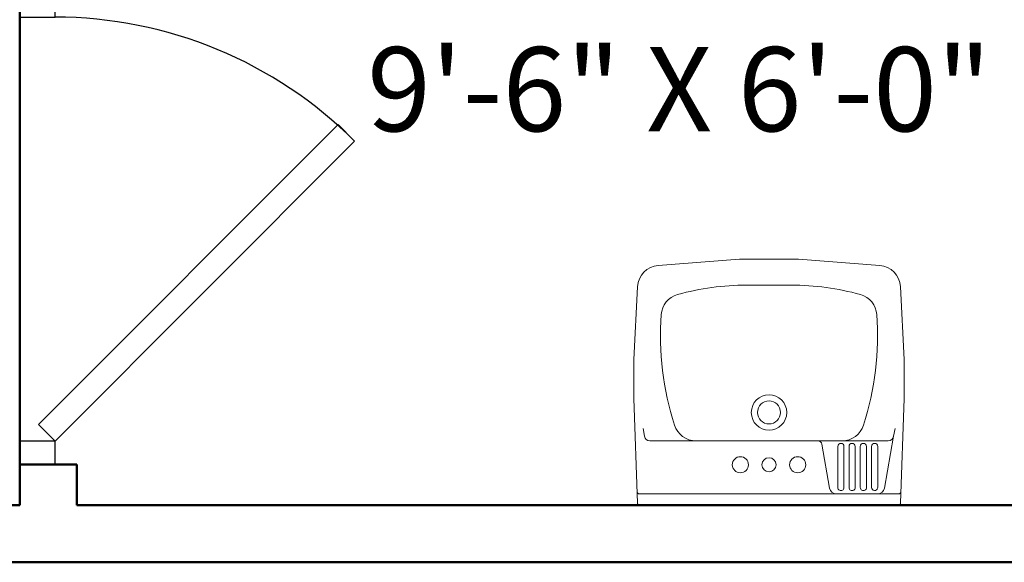
# Model space of a CAD drawing. Units: inches. Extents: x 64 to 1167, y 117 to 939.
# Tile 13 of 56: x 179 to 248, y 781 to 819. Entities that reach past the tile are written whole.
import ezdxf

# ---------------------------------------------------------------- set-up
doc = ezdxf.new("R2010")
doc.units = ezdxf.units.IN
doc.header["$MEASUREMENT"] = 0
for name, color, linetype, lineweight in [('A-ANNO-TEXT', 7, 'Continuous', 25), ('A-DOOR', 4, 'Continuous', 25), ('A-FLOR-FIXT', 8, 'Continuous', 18), ('A-WALL', 7, 'Continuous', 50)]:
    doc.layers.add(name, color=color, linetype=linetype, lineweight=lineweight)
doc.styles.get("Standard").update_dxf_attribs({"font": 'arial.ttf'})

# ---------------------------------------------------------------- blocks, each defined once
blk = doc.blocks.new('A$C68901CC0')
for p, q in [((10.955, 26.616), (12.347, 28.008)), ((12.347, 28.008), (37.402, 2.953)), ((36.01, 1.561), (10.955, 26.616)), ((0, 2.953), (0, 0)), ((1.969, 2.953), (0, 2.953)), ((1.969, 0), (1.969, 2.953)), ((37.402, 2.953), (36.01, 1.561)), ((37.402, 2.953), (37.402, 0)), ((39.37, 2.953), (37.402, 2.953)), ((39.37, 0), (39.37, 2.953)), ((0, 0), (1.969, 0)), ((37.402, 0), (39.37, 0))]:
    blk.add_line(p, q)
blk.add_arc((37.402, 2.953), 35.433, 135, 180)
blk = doc.blocks.new('A$C056A4ABE')
at = {"ltscale": 20}
for p, q in [((0.0065, 0.4339), (0, 0.2479)), ((0.2406, 0.4378), (0.0105, 0.4378)), ((0.2406, 0.4378), (0.4708, 0.4378)), ((0.4748, 0.4339), (0.4813, 0.2479)), ((0.0098, 0.4178), (0.2406, 0.4178)), ((0.0188, 0.315), (0.0351, 0.4075)), ((0.0472, 0.4063), (0.0472, 0.3333)), ((0.1205, 0.4178), (0.0475, 0.4178)), ((0.11, 0.4178), (0.0579, 0.4178)), ((0.0582, 0.4063), (0.0582, 0.3333)), ((0.0672, 0.4063), (0.0672, 0.3333)), ((0.0782, 0.4063), (0.0782, 0.3333)), ((0.0872, 0.4063), (0.0872, 0.3333)), ((0.0982, 0.4063), (0.0982, 0.3333)), ((0.1072, 0.4063), (0.1072, 0.3333)), ((0.1182, 0.4063), (0.1182, 0.3333)), ((0.1465, 0.3295), (0.1328, 0.4075)), ((0.4715, 0.4178), (0.2406, 0.4178)), ((0.2406, 0.3233), (0.0287, 0.3233)), ((0.2406, 0.3233), (0.1468, 0.3233)), ((0.2406, 0.3233), (0.3344, 0.3233)), ((0.2406, 0.3233), (0.4526, 0.3233)), ((0.0164, 0.3013), (0.0188, 0.315)), ((0.4648, 0.3013), (0.4624, 0.315)), ((0, 0.2479), (0, 0.1789)), ((0.4813, 0.2479), (0.4813, 0.1789)), ((0, 0.1789), (0.0068, 0.0492)), ((0.4813, 0.1789), (0.4745, 0.0492)), ((0.2406, 0.0463), (0.2011, 0.0463)), ((0.2406, 0.0463), (0.2802, 0.0463)), ((0.0436, 0.0114), (0.1881, 0)), ((0.1881, 0), (0.2406, 0)), ((0.2932, 0), (0.2406, 0)), ((0.4377, 0.0114), (0.2932, 0))]:
    blk.add_line(p, q, dxfattribs=at)
for centre, radius in [((0.1896, 0.3658), 0.0143), ((0.2406, 0.3658), 0.0125), ((0.2916, 0.3658), 0.0143), ((0.2406, 0.2728), 0.0315), ((0.2406, 0.2728), 0.0205)]:
    blk.add_circle(centre, radius, dxfattribs=at)
for centre, radius, start, end in [((0.0105, 0.4338), 0.004, 90, 178), ((0.4708, 0.4338), 0.004, 2, 90), ((0.0098, 0.4138), 0.004, 90, 178), ((0.0475, 0.4053), 0.0125, 90, 170), ((0.0527, 0.4063), 0.0055, 0, 172.1464), ((0.0727, 0.4063), 0.0055, 0, 180), ((0.0927, 0.4063), 0.0055, 0, 180), ((0.1127, 0.4063), 0.0055, 0, 180), ((0.1205, 0.4053), 0.0125, 10, 90), ((0.4715, 0.4138), 0.004, 2, 90), ((0.0527, 0.3333), 0.0055, 180, 0), ((0.0727, 0.3333), 0.0055, 180, 0), ((0.0927, 0.3333), 0.0055, 180, 0), ((0.1127, 0.3333), 0.0055, 180, 0), ((0.0287, 0.3133), 0.01, 90, 170), ((0.1106, 0.2833), 0.04, 90, 162.5107), ((0.1539, 0.3308), 0.0075, 190, 270), ((0.3706, 0.2833), 0.04, 17.4893, 90), ((0.4526, 0.3133), 0.01, 10, 90), ((0.5633, 0.1363), 0.516, 162.0492, 184.1817), ((-0.0821, 0.1363), 0.516, 355.8183, 17.9508), ((0.0886, 0.1016), 0.04, 184.1813, 254.5087), ((0.3926, 0.1016), 0.04, 285.4913, 355.8187), ((0.2011, 0.5073), 0.461, 254.5087, 270), ((0.2802, 0.5073), 0.461, 270, 285.4913), ((0.0467, 0.0512), 0.04, 183, 265.5), ((0.4345, 0.0512), 0.04, 274.5, 357)]:
    blk.add_arc(centre, radius, start, end, dxfattribs=at)

msp = doc.modelspace()

# ---------------------------------------------------------------- linework, layer by layer
at = {"layer": 'A-WALL'}
for p, q in [((179.107, 788.043), (179.107, 821.03)), ((183.107, 788.043), (179.107, 788.043)), ((179.107, 788.043), (179.107, 785.2)), ((183.107, 788.043), (183.107, 785.2)), ((179.107, 785.2), (166.795, 785.2)), ((297.107, 785.2), (183.107, 785.2)), ((297.107, 781.2), (166.795, 781.2))]:
    msp.add_line(p, q, dxfattribs=at)

# ---------------------------------------------------------------- block references
at = {"layer": 'A-DOOR', "xscale": 0.837864491618382, "yscale": 0.837864491618382, "zscale": 0.837864491618382, "rotation": 270}
msp.add_blockref('A$C68901CC0', (179.107, 821.03), dxfattribs=at)
at = {"layer": 'A-FLOR-FIXT', "xscale": 39.37007874015748, "yscale": 39.37007874015748, "zscale": 39.37007874015748, "rotation": 180.0000000032171}
msp.add_blockref('A$C056A4ABE', (241.075, 802.435), dxfattribs=at)

# ---------------------------------------------------------------- texts
at = {"layer": 'A-ANNO-TEXT'}
msp.add_text(' 9\'-6" X 6\'-0"', height=5.89263, dxfattribs=at).set_placement((201.648, 811.386))

doc.saveas('drawing.dxf')
